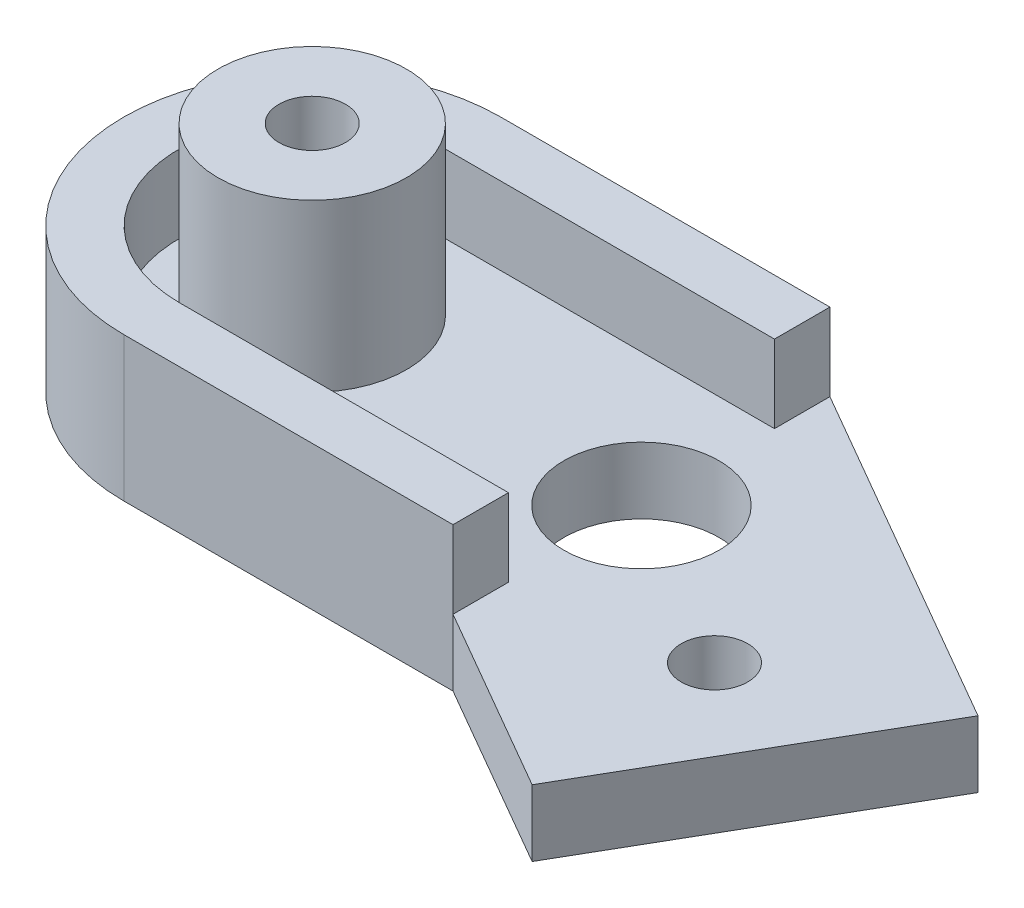
ISO-10303-21;
HEADER;
FILE_DESCRIPTION(('STEP AP214'),'2;1');
FILE_NAME('part.step','',(''),(''),'','','');
FILE_SCHEMA(('AUTOMOTIVE_DESIGN { 1 0 10303 214 1 1 1 1 }'));
ENDSEC;
DATA;
#1=APPLICATION_CONTEXT('core data for automotive mechanical design processes');
#2=APPLICATION_PROTOCOL_DEFINITION('international standard','automotive_design',2000,#1);
#3=PRODUCT_CONTEXT('',#1,'mechanical');
#4=PRODUCT('Part','Part','',(#3));
#5=PRODUCT_RELATED_PRODUCT_CATEGORY('part','',(#4));
#6=PRODUCT_DEFINITION_FORMATION('','',#4);
#7=PRODUCT_DEFINITION_CONTEXT('part definition',#1,'design');
#8=PRODUCT_DEFINITION('design','',#6,#7);
#9=PRODUCT_DEFINITION_SHAPE('','',#8);
#10=(LENGTH_UNIT() NAMED_UNIT(*) SI_UNIT(.MILLI.,.METRE.));
#11=(NAMED_UNIT(*) PLANE_ANGLE_UNIT() SI_UNIT($,.RADIAN.));
#12=(NAMED_UNIT(*) SI_UNIT($,.STERADIAN.) SOLID_ANGLE_UNIT());
#13=UNCERTAINTY_MEASURE_WITH_UNIT(LENGTH_MEASURE(1.E-05),#10,'distance_accuracy_value','');
#14=(GEOMETRIC_REPRESENTATION_CONTEXT(3) GLOBAL_UNCERTAINTY_ASSIGNED_CONTEXT((#13)) GLOBAL_UNIT_ASSIGNED_CONTEXT((#10,
#11,#12)) REPRESENTATION_CONTEXT('',''));
#15=CARTESIAN_POINT('',(0.,0.,0.));
#16=DIRECTION('',(0.,0.,1.));
#17=DIRECTION('',(1.,0.,0.));
#18=AXIS2_PLACEMENT_3D('',#15,#16,#17);
#19=CARTESIAN_POINT('',(59.4,26.,-34.));
#20=DIRECTION('',(-1.,0.,0.));
#21=DIRECTION('',(0.,0.,1.));
#22=AXIS2_PLACEMENT_3D('',#19,#20,#21);
#23=PLANE('',#22);
#24=DIRECTION('',(0.,0.,1.));
#25=VECTOR('',#24,1.);
#26=CARTESIAN_POINT('',(59.4,12.,-34.));
#27=LINE('',#26,#25);
#28=CARTESIAN_POINT('',(59.4,12.,-34.));
#29=VERTEX_POINT('',#28);
#30=CARTESIAN_POINT('',(59.4,12.,-24.));
#31=VERTEX_POINT('',#30);
#32=EDGE_CURVE('E54',#29,#31,#27,.T.);
#33=ORIENTED_EDGE('',*,*,#32,.F.);
#34=DIRECTION('',(0.,-1.,0.));
#35=VECTOR('',#34,1.);
#36=CARTESIAN_POINT('',(59.4,26.,-34.));
#37=LINE('',#36,#35);
#38=CARTESIAN_POINT('',(59.4,26.,-34.));
#39=VERTEX_POINT('',#38);
#40=EDGE_CURVE('E219',#39,#29,#37,.T.);
#41=ORIENTED_EDGE('',*,*,#40,.F.);
#42=DIRECTION('',(0.,0.,-1.));
#43=VECTOR('',#42,1.);
#44=CARTESIAN_POINT('',(59.4,26.,-34.));
#45=LINE('',#44,#43);
#46=CARTESIAN_POINT('',(59.4,26.,-24.));
#47=VERTEX_POINT('',#46);
#48=EDGE_CURVE('E206',#47,#39,#45,.T.);
#49=ORIENTED_EDGE('',*,*,#48,.F.);
#50=DIRECTION('',(0.,1.,0.));
#51=VECTOR('',#50,1.);
#52=CARTESIAN_POINT('',(59.4,12.,-24.));
#53=LINE('',#52,#51);
#54=EDGE_CURVE('E192',#31,#47,#53,.T.);
#55=ORIENTED_EDGE('',*,*,#54,.F.);
#56=EDGE_LOOP('',(#33,#41,#49,#55));
#57=FACE_BOUND('',#56,.T.);
#58=ADVANCED_FACE('F44',(#57),#23,.F.);
#59=CARTESIAN_POINT('',(59.4,12.,24.));
#60=VERTEX_POINT('',#59);
#61=CARTESIAN_POINT('',(59.4,12.,34.));
#62=VERTEX_POINT('',#61);
#63=EDGE_CURVE('E11',#60,#62,#27,.T.);
#64=ORIENTED_EDGE('',*,*,#63,.F.);
#65=DIRECTION('',(0.,1.,0.));
#66=VECTOR('',#65,1.);
#67=CARTESIAN_POINT('',(59.4,12.,24.));
#68=LINE('',#67,#66);
#69=CARTESIAN_POINT('',(59.4,26.,24.));
#70=VERTEX_POINT('',#69);
#71=EDGE_CURVE('E198',#60,#70,#68,.T.);
#72=ORIENTED_EDGE('',*,*,#71,.T.);
#73=CARTESIAN_POINT('',(59.4,26.,34.));
#74=VERTEX_POINT('',#73);
#75=EDGE_CURVE('E210',#74,#70,#45,.T.);
#76=ORIENTED_EDGE('',*,*,#75,.F.);
#77=DIRECTION('',(0.,-1.,0.));
#78=VECTOR('',#77,1.);
#79=CARTESIAN_POINT('',(59.4,26.,34.));
#80=LINE('',#79,#78);
#81=EDGE_CURVE('E222',#74,#62,#80,.T.);
#82=ORIENTED_EDGE('',*,*,#81,.T.);
#83=EDGE_LOOP('',(#64,#72,#76,#82));
#84=FACE_BOUND('',#83,.T.);
#85=ADVANCED_FACE('F238',(#84),#23,.F.);
#86=CARTESIAN_POINT('',(0.,26.,0.));
#87=DIRECTION('',(0.,-1.,0.));
#88=DIRECTION('',(0.,0.,-1.));
#89=AXIS2_PLACEMENT_3D('',#86,#87,#88);
#90=CYLINDRICAL_SURFACE('',#89,34.);
#91=CARTESIAN_POINT('',(0.,0.,0.));
#92=DIRECTION('',(0.,1.,0.));
#93=DIRECTION('',(0.,0.,1.));
#94=AXIS2_PLACEMENT_3D('',#91,#92,#93);
#95=CIRCLE('',#94,34.);
#96=CARTESIAN_POINT('',(0.,0.,-34.));
#97=VERTEX_POINT('',#96);
#98=CARTESIAN_POINT('',(0.,0.,34.));
#99=VERTEX_POINT('',#98);
#100=EDGE_CURVE('E191',#97,#99,#95,.T.);
#101=ORIENTED_EDGE('',*,*,#100,.T.);
#102=DIRECTION('',(0.,-1.,0.));
#103=VECTOR('',#102,1.);
#104=CARTESIAN_POINT('',(0.,26.,34.));
#105=LINE('',#104,#103);
#106=CARTESIAN_POINT('',(0.,26.,34.));
#107=VERTEX_POINT('',#106);
#108=EDGE_CURVE('E47',#107,#99,#105,.T.);
#109=ORIENTED_EDGE('',*,*,#108,.F.);
#110=CARTESIAN_POINT('',(0.,26.,0.));
#111=DIRECTION('',(0.,1.,0.));
#112=DIRECTION('',(0.,0.,1.));
#113=AXIS2_PLACEMENT_3D('',#110,#111,#112);
#114=CIRCLE('',#113,34.);
#115=CARTESIAN_POINT('',(0.,26.,-34.));
#116=VERTEX_POINT('',#115);
#117=EDGE_CURVE('E199',#116,#107,#114,.T.);
#118=ORIENTED_EDGE('',*,*,#117,.F.);
#119=DIRECTION('',(0.,-1.,0.));
#120=VECTOR('',#119,1.);
#121=CARTESIAN_POINT('',(0.,26.,-34.));
#122=LINE('',#121,#120);
#123=EDGE_CURVE('E215',#116,#97,#122,.T.);
#124=ORIENTED_EDGE('',*,*,#123,.T.);
#125=EDGE_LOOP('',(#101,#109,#118,#124));
#126=FACE_BOUND('',#125,.T.);
#127=ADVANCED_FACE('F50',(#126),#90,.T.);
#128=CARTESIAN_POINT('',(59.4,26.,34.));
#129=DIRECTION('',(0.,0.,-1.));
#130=DIRECTION('',(-1.,0.,0.));
#131=AXIS2_PLACEMENT_3D('',#128,#129,#130);
#132=PLANE('',#131);
#133=DIRECTION('',(1.,0.,0.));
#134=VECTOR('',#133,1.);
#135=CARTESIAN_POINT('',(59.4,0.,34.));
#136=LINE('',#135,#134);
#137=CARTESIAN_POINT('',(59.4,0.,34.));
#138=VERTEX_POINT('',#137);
#139=EDGE_CURVE('E214',#99,#138,#136,.T.);
#140=ORIENTED_EDGE('',*,*,#139,.T.);
#141=DIRECTION('',(0.,1.,0.));
#142=VECTOR('',#141,1.);
#143=CARTESIAN_POINT('',(59.4,0.,34.));
#144=LINE('',#143,#142);
#145=EDGE_CURVE('E141',#138,#62,#144,.T.);
#146=ORIENTED_EDGE('',*,*,#145,.T.);
#147=ORIENTED_EDGE('',*,*,#81,.F.);
#148=DIRECTION('',(1.,0.,0.));
#149=VECTOR('',#148,1.);
#150=CARTESIAN_POINT('',(59.4,26.,34.));
#151=LINE('',#150,#149);
#152=EDGE_CURVE('E201',#107,#74,#151,.T.);
#153=ORIENTED_EDGE('',*,*,#152,.F.);
#154=ORIENTED_EDGE('',*,*,#108,.T.);
#155=EDGE_LOOP('',(#140,#146,#147,#153,#154));
#156=FACE_BOUND('',#155,.T.);
#157=ADVANCED_FACE('F227',(#156),#132,.F.);
#158=CARTESIAN_POINT('',(0.,26.,-34.));
#159=DIRECTION('',(0.,0.,1.));
#160=DIRECTION('',(1.,0.,0.));
#161=AXIS2_PLACEMENT_3D('',#158,#159,#160);
#162=PLANE('',#161);
#163=DIRECTION('',(-1.,0.,0.));
#164=VECTOR('',#163,1.);
#165=CARTESIAN_POINT('',(0.,0.,-34.));
#166=LINE('',#165,#164);
#167=CARTESIAN_POINT('',(59.4,0.,-34.));
#168=VERTEX_POINT('',#167);
#169=EDGE_CURVE('E204',#168,#97,#166,.T.);
#170=ORIENTED_EDGE('',*,*,#169,.T.);
#171=ORIENTED_EDGE('',*,*,#123,.F.);
#172=DIRECTION('',(-1.,0.,0.));
#173=VECTOR('',#172,1.);
#174=CARTESIAN_POINT('',(0.,26.,-34.));
#175=LINE('',#174,#173);
#176=EDGE_CURVE('E209',#39,#116,#175,.T.);
#177=ORIENTED_EDGE('',*,*,#176,.F.);
#178=ORIENTED_EDGE('',*,*,#40,.T.);
#179=DIRECTION('',(0.,1.,0.));
#180=VECTOR('',#179,1.);
#181=CARTESIAN_POINT('',(59.4,0.,-34.));
#182=LINE('',#181,#180);
#183=EDGE_CURVE('E168',#168,#29,#182,.T.);
#184=ORIENTED_EDGE('',*,*,#183,.F.);
#185=EDGE_LOOP('',(#170,#171,#177,#178,#184));
#186=FACE_BOUND('',#185,.T.);
#187=ADVANCED_FACE('F247',(#186),#162,.F.);
#188=CARTESIAN_POINT('',(0.,26.,0.));
#189=DIRECTION('',(0.,1.,0.));
#190=DIRECTION('',(0.,0.,1.));
#191=AXIS2_PLACEMENT_3D('',#188,#189,#190);
#192=PLANE('',#191);
#193=DIRECTION('',(-1.,0.,0.));
#194=VECTOR('',#193,1.);
#195=CARTESIAN_POINT('',(0.,26.,-24.));
#196=LINE('',#195,#194);
#197=CARTESIAN_POINT('',(0.,26.,-24.));
#198=VERTEX_POINT('',#197);
#199=EDGE_CURVE('E177',#47,#198,#196,.T.);
#200=ORIENTED_EDGE('',*,*,#199,.F.);
#201=ORIENTED_EDGE('',*,*,#48,.T.);
#202=ORIENTED_EDGE('',*,*,#176,.T.);
#203=ORIENTED_EDGE('',*,*,#117,.T.);
#204=ORIENTED_EDGE('',*,*,#152,.T.);
#205=ORIENTED_EDGE('',*,*,#75,.T.);
#206=DIRECTION('',(1.,0.,0.));
#207=VECTOR('',#206,1.);
#208=CARTESIAN_POINT('',(59.4,26.,24.));
#209=LINE('',#208,#207);
#210=CARTESIAN_POINT('',(0.,26.,24.));
#211=VERTEX_POINT('',#210);
#212=EDGE_CURVE('E190',#211,#70,#209,.T.);
#213=ORIENTED_EDGE('',*,*,#212,.F.);
#214=CARTESIAN_POINT('',(0.,26.,0.));
#215=DIRECTION('',(0.,1.,0.));
#216=DIRECTION('',(0.,0.,1.));
#217=AXIS2_PLACEMENT_3D('',#214,#215,#216);
#218=CIRCLE('',#217,24.);
#219=EDGE_CURVE('E67',#198,#211,#218,.T.);
#220=ORIENTED_EDGE('',*,*,#219,.F.);
#221=EDGE_LOOP('',(#200,#201,#202,#203,#204,#205,#213,#220));
#222=FACE_BOUND('',#221,.T.);
#223=ADVANCED_FACE('F248',(#222),#192,.T.);
#224=CARTESIAN_POINT('',(0.,0.,0.));
#225=DIRECTION('',(0.,1.,0.));
#226=DIRECTION('',(0.,0.,1.));
#227=AXIS2_PLACEMENT_3D('',#224,#225,#226);
#228=PLANE('',#227);
#229=CARTESIAN_POINT('',(59.4,0.,0.));
#230=DIRECTION('',(0.,1.,0.));
#231=DIRECTION('',(0.,0.,1.));
#232=AXIS2_PLACEMENT_3D('',#229,#230,#231);
#233=CIRCLE('',#232,14.);
#234=CARTESIAN_POINT('',(59.4,0.,14.));
#235=VERTEX_POINT('',#234);
#236=EDGE_CURVE('E436',#235,#235,#233,.T.);
#237=ORIENTED_EDGE('',*,*,#236,.T.);
#238=EDGE_LOOP('',(#237));
#239=FACE_BOUND('',#238,.T.);
#240=CARTESIAN_POINT('',(90.5769145362398,0.,18.));
#241=DIRECTION('',(0.,1.,0.));
#242=DIRECTION('',(0.,0.,1.));
#243=AXIS2_PLACEMENT_3D('',#240,#241,#242);
#244=CIRCLE('',#243,6.);
#245=CARTESIAN_POINT('',(90.5769145362398,0.,24.));
#246=VERTEX_POINT('',#245);
#247=EDGE_CURVE('E442',#246,#246,#244,.T.);
#248=ORIENTED_EDGE('',*,*,#247,.T.);
#249=EDGE_LOOP('',(#248));
#250=FACE_BOUND('',#249,.T.);
#251=CARTESIAN_POINT('',(0.,0.,0.));
#252=DIRECTION('',(0.,1.,0.));
#253=DIRECTION('',(0.,0.,1.));
#254=AXIS2_PLACEMENT_3D('',#251,#252,#253);
#255=CIRCLE('',#254,6.);
#256=CARTESIAN_POINT('',(0.,0.,6.));
#257=VERTEX_POINT('',#256);
#258=EDGE_CURVE('E429',#257,#257,#255,.T.);
#259=ORIENTED_EDGE('',*,*,#258,.T.);
#260=EDGE_LOOP('',(#259));
#261=FACE_BOUND('',#260,.T.);
#262=ORIENTED_EDGE('',*,*,#100,.F.);
#263=ORIENTED_EDGE('',*,*,#169,.F.);
#264=DIRECTION('',(-0.866025403784438,0.,-0.500000000000001));
#265=VECTOR('',#264,1.);
#266=CARTESIAN_POINT('',(59.4,0.,-34.));
#267=LINE('',#266,#265);
#268=CARTESIAN_POINT('',(122.619854476264,0.,2.50000000000008));
#269=VERTEX_POINT('',#268);
#270=EDGE_CURVE('E155',#269,#168,#267,.T.);
#271=ORIENTED_EDGE('',*,*,#270,.F.);
#272=DIRECTION('',(0.500000000000001,0.,-0.866025403784438));
#273=VECTOR('',#272,1.);
#274=CARTESIAN_POINT('',(122.619854476264,0.,2.50000000000008));
#275=LINE('',#274,#273);
#276=CARTESIAN_POINT('',(93.174990747593,0.,53.5));
#277=VERTEX_POINT('',#276);
#278=EDGE_CURVE('E133',#277,#269,#275,.T.);
#279=ORIENTED_EDGE('',*,*,#278,.F.);
#280=DIRECTION('',(0.866025403784438,0.,0.500000000000001));
#281=VECTOR('',#280,1.);
#282=CARTESIAN_POINT('',(59.4,0.,34.));
#283=LINE('',#282,#281);
#284=EDGE_CURVE('E149',#138,#277,#283,.T.);
#285=ORIENTED_EDGE('',*,*,#284,.F.);
#286=ORIENTED_EDGE('',*,*,#139,.F.);
#287=EDGE_LOOP('',(#262,#263,#271,#279,#285,#286));
#288=FACE_BOUND('',#287,.T.);
#289=ADVANCED_FACE('F146',(#239,#250,#261,#288),#228,.F.);
#290=CARTESIAN_POINT('',(0.,12.,0.));
#291=DIRECTION('',(0.,1.,0.));
#292=DIRECTION('',(0.,0.,1.));
#293=AXIS2_PLACEMENT_3D('',#290,#291,#292);
#294=CYLINDRICAL_SURFACE('',#293,24.);
#295=ORIENTED_EDGE('',*,*,#219,.T.);
#296=DIRECTION('',(0.,1.,0.));
#297=VECTOR('',#296,1.);
#298=CARTESIAN_POINT('',(0.,12.,24.));
#299=LINE('',#298,#297);
#300=CARTESIAN_POINT('',(0.,12.,24.));
#301=VERTEX_POINT('',#300);
#302=EDGE_CURVE('E183',#301,#211,#299,.T.);
#303=ORIENTED_EDGE('',*,*,#302,.F.);
#304=CARTESIAN_POINT('',(0.,12.,0.));
#305=DIRECTION('',(0.,1.,0.));
#306=DIRECTION('',(0.,0.,1.));
#307=AXIS2_PLACEMENT_3D('',#304,#305,#306);
#308=CIRCLE('',#307,24.);
#309=CARTESIAN_POINT('',(0.,12.,-24.));
#310=VERTEX_POINT('',#309);
#311=EDGE_CURVE('E174',#310,#301,#308,.T.);
#312=ORIENTED_EDGE('',*,*,#311,.F.);
#313=DIRECTION('',(0.,1.,0.));
#314=VECTOR('',#313,1.);
#315=CARTESIAN_POINT('',(0.,12.,-24.));
#316=LINE('',#315,#314);
#317=EDGE_CURVE('E193',#310,#198,#316,.T.);
#318=ORIENTED_EDGE('',*,*,#317,.T.);
#319=EDGE_LOOP('',(#295,#303,#312,#318));
#320=FACE_BOUND('',#319,.T.);
#321=ADVANCED_FACE('F278',(#320),#294,.F.);
#322=CARTESIAN_POINT('',(0.,12.,-24.));
#323=DIRECTION('',(0.,0.,-1.));
#324=DIRECTION('',(-1.,0.,0.));
#325=AXIS2_PLACEMENT_3D('',#322,#323,#324);
#326=PLANE('',#325);
#327=ORIENTED_EDGE('',*,*,#199,.T.);
#328=ORIENTED_EDGE('',*,*,#317,.F.);
#329=DIRECTION('',(-1.,0.,0.));
#330=VECTOR('',#329,1.);
#331=CARTESIAN_POINT('',(0.,12.,-24.));
#332=LINE('',#331,#330);
#333=EDGE_CURVE('E185',#31,#310,#332,.T.);
#334=ORIENTED_EDGE('',*,*,#333,.F.);
#335=ORIENTED_EDGE('',*,*,#54,.T.);
#336=EDGE_LOOP('',(#327,#328,#334,#335));
#337=FACE_BOUND('',#336,.T.);
#338=ADVANCED_FACE('F282',(#337),#326,.F.);
#339=CARTESIAN_POINT('',(59.4,12.,24.));
#340=DIRECTION('',(0.,0.,1.));
#341=DIRECTION('',(1.,0.,0.));
#342=AXIS2_PLACEMENT_3D('',#339,#340,#341);
#343=PLANE('',#342);
#344=ORIENTED_EDGE('',*,*,#212,.T.);
#345=ORIENTED_EDGE('',*,*,#71,.F.);
#346=DIRECTION('',(1.,0.,0.));
#347=VECTOR('',#346,1.);
#348=CARTESIAN_POINT('',(59.4,12.,24.));
#349=LINE('',#348,#347);
#350=EDGE_CURVE('E176',#301,#60,#349,.T.);
#351=ORIENTED_EDGE('',*,*,#350,.F.);
#352=ORIENTED_EDGE('',*,*,#302,.T.);
#353=EDGE_LOOP('',(#344,#345,#351,#352));
#354=FACE_BOUND('',#353,.T.);
#355=ADVANCED_FACE('F245',(#354),#343,.F.);
#356=CARTESIAN_POINT('',(0.,12.,0.));
#357=DIRECTION('',(0.,1.,0.));
#358=DIRECTION('',(0.,0.,1.));
#359=AXIS2_PLACEMENT_3D('',#356,#357,#358);
#360=PLANE('',#359);
#361=CARTESIAN_POINT('',(59.4,12.,0.));
#362=DIRECTION('',(0.,1.,0.));
#363=DIRECTION('',(0.,0.,1.));
#364=AXIS2_PLACEMENT_3D('',#361,#362,#363);
#365=CIRCLE('',#364,14.);
#366=CARTESIAN_POINT('',(59.4,12.,14.));
#367=VERTEX_POINT('',#366);
#368=EDGE_CURVE('E441',#367,#367,#365,.T.);
#369=ORIENTED_EDGE('',*,*,#368,.F.);
#370=EDGE_LOOP('',(#369));
#371=FACE_BOUND('',#370,.T.);
#372=CARTESIAN_POINT('',(90.5769145362398,12.,18.));
#373=DIRECTION('',(0.,1.,0.));
#374=DIRECTION('',(0.,0.,1.));
#375=AXIS2_PLACEMENT_3D('',#372,#373,#374);
#376=CIRCLE('',#375,6.);
#377=CARTESIAN_POINT('',(90.5769145362398,12.,24.));
#378=VERTEX_POINT('',#377);
#379=EDGE_CURVE('E443',#378,#378,#376,.T.);
#380=ORIENTED_EDGE('',*,*,#379,.F.);
#381=EDGE_LOOP('',(#380));
#382=FACE_BOUND('',#381,.T.);
#383=CARTESIAN_POINT('',(0.,12.,0.));
#384=DIRECTION('',(0.,1.,0.));
#385=DIRECTION('',(0.,0.,1.));
#386=AXIS2_PLACEMENT_3D('',#383,#384,#385);
#387=CIRCLE('',#386,17.);
#388=CARTESIAN_POINT('',(0.,12.,17.));
#389=VERTEX_POINT('',#388);
#390=EDGE_CURVE('E165',#389,#389,#387,.T.);
#391=ORIENTED_EDGE('',*,*,#390,.F.);
#392=EDGE_LOOP('',(#391));
#393=FACE_BOUND('',#392,.T.);
#394=ORIENTED_EDGE('',*,*,#311,.T.);
#395=ORIENTED_EDGE('',*,*,#350,.T.);
#396=ORIENTED_EDGE('',*,*,#63,.T.);
#397=DIRECTION('',(0.866025403784438,0.,0.500000000000001));
#398=VECTOR('',#397,1.);
#399=CARTESIAN_POINT('',(59.4,12.,34.));
#400=LINE('',#399,#398);
#401=CARTESIAN_POINT('',(93.174990747593,12.,53.5));
#402=VERTEX_POINT('',#401);
#403=EDGE_CURVE('E167',#62,#402,#400,.T.);
#404=ORIENTED_EDGE('',*,*,#403,.T.);
#405=DIRECTION('',(0.500000000000001,0.,-0.866025403784438));
#406=VECTOR('',#405,1.);
#407=CARTESIAN_POINT('',(122.619854476264,12.,2.50000000000008));
#408=LINE('',#407,#406);
#409=CARTESIAN_POINT('',(122.619854476264,12.,2.50000000000008));
#410=VERTEX_POINT('',#409);
#411=EDGE_CURVE('E140',#402,#410,#408,.T.);
#412=ORIENTED_EDGE('',*,*,#411,.T.);
#413=DIRECTION('',(-0.866025403784438,0.,-0.500000000000001));
#414=VECTOR('',#413,1.);
#415=CARTESIAN_POINT('',(59.4,12.,-34.));
#416=LINE('',#415,#414);
#417=EDGE_CURVE('E160',#410,#29,#416,.T.);
#418=ORIENTED_EDGE('',*,*,#417,.T.);
#419=ORIENTED_EDGE('',*,*,#32,.T.);
#420=ORIENTED_EDGE('',*,*,#333,.T.);
#421=EDGE_LOOP('',(#394,#395,#396,#404,#412,#418,#419,#420));
#422=FACE_BOUND('',#421,.T.);
#423=ADVANCED_FACE('F240',(#371,#382,#393,#422),#360,.T.);
#424=CARTESIAN_POINT('',(59.4,0.,-34.));
#425=DIRECTION('',(0.500000000000001,0.,-0.866025403784438));
#426=DIRECTION('',(-0.866025403784438,0.,-0.500000000000001));
#427=AXIS2_PLACEMENT_3D('',#424,#425,#426);
#428=PLANE('',#427);
#429=ORIENTED_EDGE('',*,*,#417,.F.);
#430=DIRECTION('',(0.,1.,0.));
#431=VECTOR('',#430,1.);
#432=CARTESIAN_POINT('',(122.619854476264,0.,2.50000000000008));
#433=LINE('',#432,#431);
#434=EDGE_CURVE('E142',#269,#410,#433,.T.);
#435=ORIENTED_EDGE('',*,*,#434,.F.);
#436=ORIENTED_EDGE('',*,*,#270,.T.);
#437=ORIENTED_EDGE('',*,*,#183,.T.);
#438=EDGE_LOOP('',(#429,#435,#436,#437));
#439=FACE_BOUND('',#438,.T.);
#440=ADVANCED_FACE('F234',(#439),#428,.T.);
#441=CARTESIAN_POINT('',(122.619854476264,0.,2.50000000000008));
#442=DIRECTION('',(0.866025403784438,0.,0.500000000000001));
#443=DIRECTION('',(0.500000000000001,0.,-0.866025403784438));
#444=AXIS2_PLACEMENT_3D('',#441,#442,#443);
#445=PLANE('',#444);
#446=ORIENTED_EDGE('',*,*,#411,.F.);
#447=DIRECTION('',(0.,1.,0.));
#448=VECTOR('',#447,1.);
#449=CARTESIAN_POINT('',(93.174990747593,0.,53.5));
#450=LINE('',#449,#448);
#451=EDGE_CURVE('E131',#277,#402,#450,.T.);
#452=ORIENTED_EDGE('',*,*,#451,.F.);
#453=ORIENTED_EDGE('',*,*,#278,.T.);
#454=ORIENTED_EDGE('',*,*,#434,.T.);
#455=EDGE_LOOP('',(#446,#452,#453,#454));
#456=FACE_BOUND('',#455,.T.);
#457=ADVANCED_FACE('F132',(#456),#445,.T.);
#458=CARTESIAN_POINT('',(59.4,0.,34.));
#459=DIRECTION('',(-0.500000000000001,0.,0.866025403784438));
#460=DIRECTION('',(0.866025403784438,0.,0.500000000000001));
#461=AXIS2_PLACEMENT_3D('',#458,#459,#460);
#462=PLANE('',#461);
#463=ORIENTED_EDGE('',*,*,#403,.F.);
#464=ORIENTED_EDGE('',*,*,#145,.F.);
#465=ORIENTED_EDGE('',*,*,#284,.T.);
#466=ORIENTED_EDGE('',*,*,#451,.T.);
#467=EDGE_LOOP('',(#463,#464,#465,#466));
#468=FACE_BOUND('',#467,.T.);
#469=ADVANCED_FACE('F154',(#468),#462,.T.);
#470=CARTESIAN_POINT('',(0.,42.,0.));
#471=DIRECTION('',(0.,-1.,0.));
#472=DIRECTION('',(0.,0.,-1.));
#473=AXIS2_PLACEMENT_3D('',#470,#471,#472);
#474=CYLINDRICAL_SURFACE('',#473,17.);
#475=CARTESIAN_POINT('',(0.,42.,0.));
#476=DIRECTION('',(0.,1.,0.));
#477=DIRECTION('',(0.,0.,1.));
#478=AXIS2_PLACEMENT_3D('',#475,#476,#477);
#479=CIRCLE('',#478,17.);
#480=CARTESIAN_POINT('',(0.,42.,17.));
#481=VERTEX_POINT('',#480);
#482=EDGE_CURVE('E170',#481,#481,#479,.T.);
#483=ORIENTED_EDGE('',*,*,#482,.F.);
#484=EDGE_LOOP('',(#483));
#485=FACE_BOUND('',#484,.T.);
#486=ORIENTED_EDGE('',*,*,#390,.T.);
#487=EDGE_LOOP('',(#486));
#488=FACE_BOUND('',#487,.T.);
#489=ADVANCED_FACE('F380',(#485,#488),#474,.T.);
#490=CARTESIAN_POINT('',(0.,42.,0.));
#491=DIRECTION('',(0.,1.,0.));
#492=DIRECTION('',(0.,0.,1.));
#493=AXIS2_PLACEMENT_3D('',#490,#491,#492);
#494=PLANE('',#493);
#495=CARTESIAN_POINT('',(0.,42.,0.));
#496=DIRECTION('',(0.,1.,0.));
#497=DIRECTION('',(0.,0.,1.));
#498=AXIS2_PLACEMENT_3D('',#495,#496,#497);
#499=CIRCLE('',#498,6.);
#500=CARTESIAN_POINT('',(0.,42.,6.));
#501=VERTEX_POINT('',#500);
#502=EDGE_CURVE('E435',#501,#501,#499,.T.);
#503=ORIENTED_EDGE('',*,*,#502,.F.);
#504=EDGE_LOOP('',(#503));
#505=FACE_BOUND('',#504,.T.);
#506=ORIENTED_EDGE('',*,*,#482,.T.);
#507=EDGE_LOOP('',(#506));
#508=FACE_BOUND('',#507,.T.);
#509=ADVANCED_FACE('F375',(#505,#508),#494,.T.);
#510=CARTESIAN_POINT('',(0.,0.,0.));
#511=DIRECTION('',(0.,1.,0.));
#512=DIRECTION('',(0.,0.,1.));
#513=AXIS2_PLACEMENT_3D('',#510,#511,#512);
#514=CYLINDRICAL_SURFACE('',#513,6.);
#515=ORIENTED_EDGE('',*,*,#258,.F.);
#516=EDGE_LOOP('',(#515));
#517=FACE_BOUND('',#516,.T.);
#518=ORIENTED_EDGE('',*,*,#502,.T.);
#519=EDGE_LOOP('',(#518));
#520=FACE_BOUND('',#519,.T.);
#521=ADVANCED_FACE('F340',(#517,#520),#514,.F.);
#522=CARTESIAN_POINT('',(90.5769145362398,-18.,18.));
#523=DIRECTION('',(0.,1.,0.));
#524=DIRECTION('',(0.,0.,1.));
#525=AXIS2_PLACEMENT_3D('',#522,#523,#524);
#526=CYLINDRICAL_SURFACE('',#525,6.);
#527=ORIENTED_EDGE('',*,*,#379,.T.);
#528=EDGE_LOOP('',(#527));
#529=FACE_BOUND('',#528,.T.);
#530=ORIENTED_EDGE('',*,*,#247,.F.);
#531=EDGE_LOOP('',(#530));
#532=FACE_BOUND('',#531,.T.);
#533=ADVANCED_FACE('F342',(#529,#532),#526,.F.);
#534=CARTESIAN_POINT('',(59.4,-18.,0.));
#535=DIRECTION('',(0.,1.,0.));
#536=DIRECTION('',(0.,0.,1.));
#537=AXIS2_PLACEMENT_3D('',#534,#535,#536);
#538=CYLINDRICAL_SURFACE('',#537,14.);
#539=ORIENTED_EDGE('',*,*,#368,.T.);
#540=EDGE_LOOP('',(#539));
#541=FACE_BOUND('',#540,.T.);
#542=ORIENTED_EDGE('',*,*,#236,.F.);
#543=EDGE_LOOP('',(#542));
#544=FACE_BOUND('',#543,.T.);
#545=ADVANCED_FACE('F348',(#541,#544),#538,.F.);
#546=CLOSED_SHELL('',(#58,#85,#127,#157,#187,#223,#289,#321,#338,#355,#423,#440,#457,#469,#489,
#509,#521,#533,#545));
#547=MANIFOLD_SOLID_BREP('B2',#546);
#548=ADVANCED_BREP_SHAPE_REPRESENTATION('',(#18,#547),#14);
#549=SHAPE_DEFINITION_REPRESENTATION(#9,#548);
ENDSEC;
END-ISO-10303-21;
